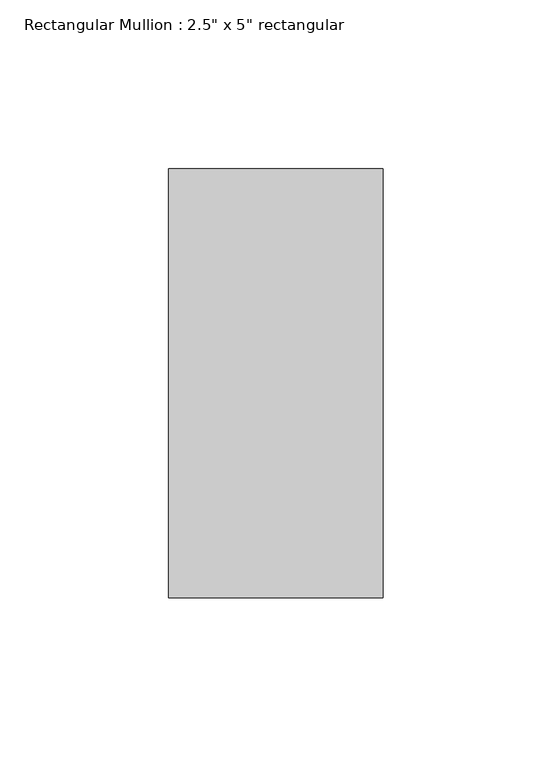
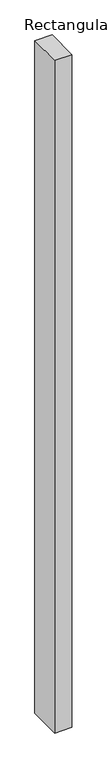
"""IFC4 building model written with IfcOpenShell, lengths in millimetres: member geometry."""

from ifc_helpers import new_model, si_unit, frame, origin, place, context, project, spatial, polyline, outline, extrude, source, transform, mapped, element, save


def member_3f28283e(model_context):
    return source(origin(), model_context, "Body", "SweptSolid", [
        extrude(outline(polyline([(0.0, 63.5), (0.0, -63.5), (-63.5, -63.5), (-63.5, 63.5), (0.0, 63.5)])), frame((0.0, 0.0, -2641.6), z_axis=(0.0, 0.0, 1.0), x_axis=(1.0, 0.0, 0.0)), (0.0, 0.0, 1.0), 2641.6),
    ])


if __name__ == "__main__":
    model = new_model("IFC4")
    model_context = context("Model", 3, world=origin())
    ifc_project = project(units=[si_unit("LENGTHUNIT", "METRE", prefix="MILLI")], contexts=[model_context])
    site = spatial("IfcSite", under=ifc_project)
    building = spatial("IfcBuilding", under=site)
    placement = place(None, origin())
    member_shape = member_3f28283e(model_context)
    element("IfcMember", 1, ObjectType="Rectangular Mullion : 2.5\" x 5\" rectangular", at=placement, inside=building, context=model_context, shape_type="MappedRepresentation", body=[
        mapped(member_shape, transform((0.0, 0.0, 0.0), x_axis=(1.0, 0.0, 0.0), y_axis=(0.0, 1.0, 0.0), z_axis=(0.0, 0.0, 1.0))),
    ])
    save(model, "model.ifc")

# Revit data of these elements
# Type "Rectangular Mullion : 2.5\" x 5\" rectangular"
#   built-in parameter 1007304 = 0.416667 (stored number, unit not read)
#   built-in parameter 1007301 = 0.104167 (stored number, unit not read)
#   built-in parameter 1007300 = 0.104167 (stored number, unit not read)
# Element 1 (IfcMember, "Rectangular Mullion : 2.5\" x 5\" rectangular")
#   Materials on its faces: "Aluminum"
# Materials
#   "Aluminum": class "Metal", colour RGB 247 247 247, transparency 0, Description = "Aluminum 6061", Cost = 0
